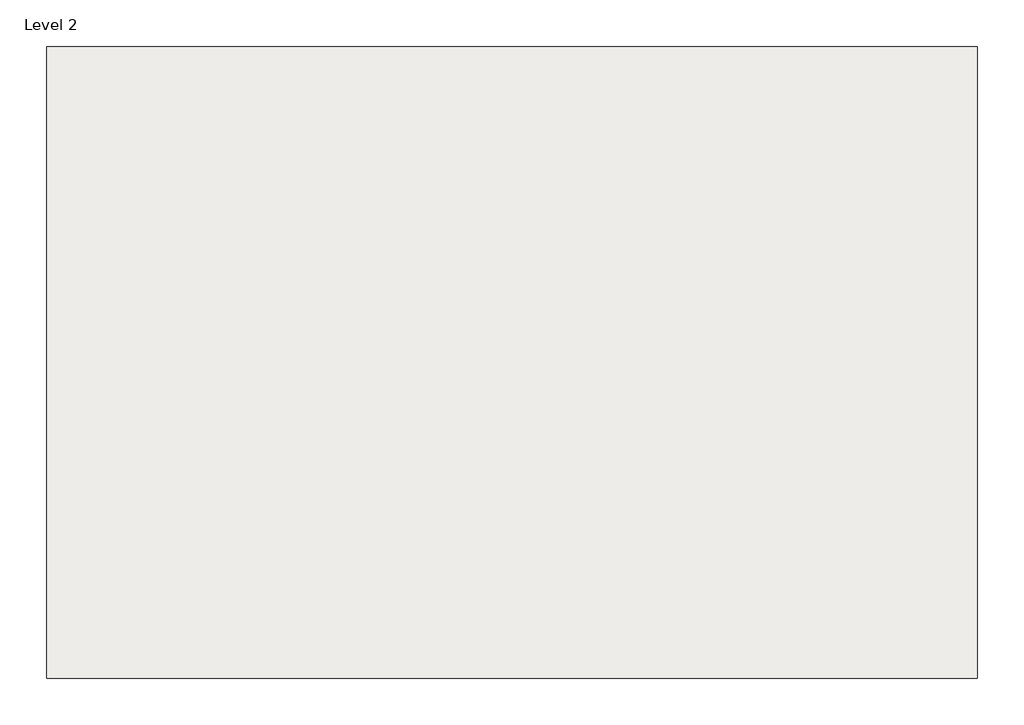
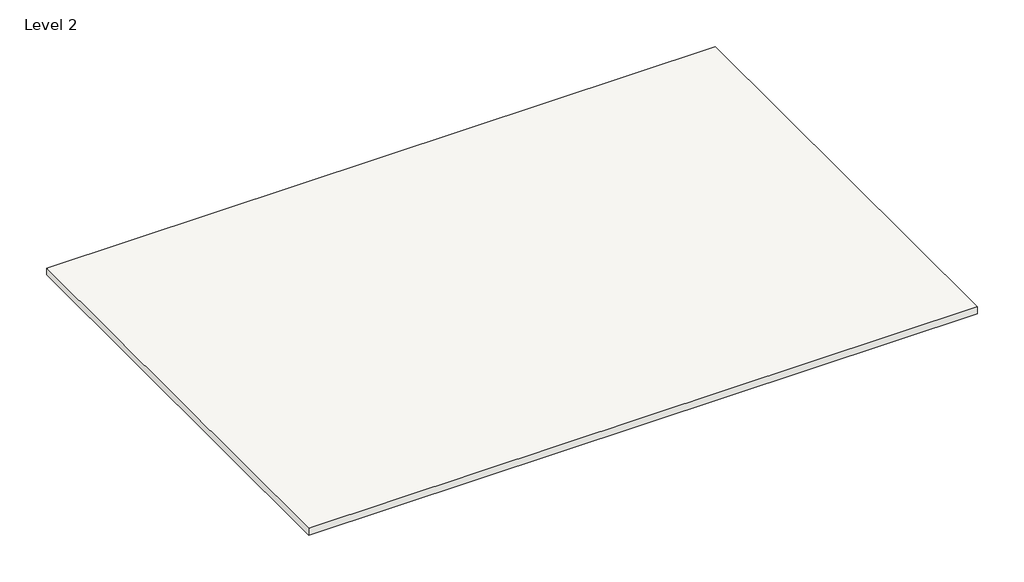
# One storey, incomplete: 1 roof.
"""IFC4 building model written with IfcOpenShell, lengths in millimetres."""

from ifc_helpers import new_model, si_unit, frame, origin, place, context, project, spatial, polyline, outline, extrude, element, save

model = new_model("IFC4")

# Units and contexts
model_context = context("Model", 3, world=origin())
ifc_project = project(units=[si_unit("LENGTHUNIT", "METRE", prefix="MILLI")], contexts=[model_context])

# Site, building, storey
site = spatial("IfcSite", under=ifc_project)
building = spatial("IfcBuilding", under=site)
storey = spatial("IfcBuildingStorey", under=building, Name="Level 2", Elevation=3048.0)

# Roof
placement = place(None, origin())
element("IfcRoof", 1, ObjectType="Generic - 12\"", at=placement, inside=storey, context=model_context, shape_type="SweptSolid", body=[
    extrude(outline(polyline([(-8134.338363, 7846.5266064), (6077.748676, 7846.5266064), (6077.748676, -1794.1868249), (-8134.338363, -1794.1868249), (-8134.338363, 7846.5266064)])), frame((0.0, 0.0, 3048.0), z_axis=(0.0, 0.0, 1.0), x_axis=(1.0, 0.0, 0.0)), (0.0, 0.0, 1.0), 152.4),
])

save(model, "model.ifc")

# Revit data of these elements
# Type "Generic - 12\""
#   Assembly Code = "B1020"
#   Layers, outside or top first: 0' - 6" no material (function 1)
# Element 1 (IfcRoof, "Generic - 12\"")
#   built-in parameter 1001705 = 10.5 (stored number, unit not read)
#   built-in parameter 1001710 = 33615
#   Phase Created = New Construction
#   Materials on its faces: "Default Roof"
# Materials
#   "Default Roof": colour RGB 88 101 114, transparency 0, Cost = 0
